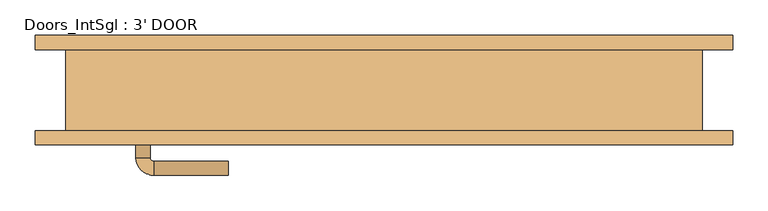
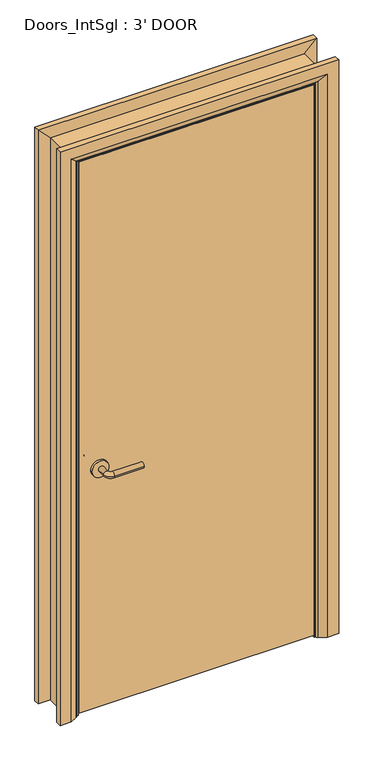
"""IFC4 building model written with IfcOpenShell, lengths in millimetres: door geometry, Doors_IntSgl : 3' DOOR."""

from ifc_helpers import new_model, si_unit, point, frame, frame_2d, origin, place, context, project, spatial, polyline, circle_curve, ellipse_curve, trimmed, segment, composite_curve, outline, extrude, faceted_brep, source, transform, mapped, element, save
from ifc_brep_helpers import plane_surface, cylinder_surface, revolved_surface, advanced_brep


def doors_intsgl_3_door_d2de26da(model_context):
    return source(origin(), model_context, "Body", "SolidModel", [
        advanced_brep(
        [(-350.2, -11.15, 900.0), (-330.2, -11.15, 900.0), (-350.2, 18.85, 900.0), (-330.2, 18.85, 900.0), (-325.2, 23.85, 900.0), (-325.2, 43.85, 900.0), (-220.2, 43.85, 900.0), (-220.2, 23.85, 900.0)],
        [
            (0, 1, circle_curve(frame((-340.2, -11.15, 900.0), z_axis=(0.0, -1.0, 0.0), x_axis=(1.0, 0.0, 0.0)), 10.0)),
            (1, 0, circle_curve(frame((-340.2, -11.15, 900.0), z_axis=(0.0, -1.0, 0.0), x_axis=(1.0, 0.0, 0.0)), 10.0)),
            (0, 2),
            (2, 3, circle_curve(frame((-340.2, 18.85, 900.0), z_axis=(0.0, -1.0, 0.0), x_axis=(1.0, 0.0, 0.0)), 10.0)),
            (3, 1),
            (3, 2, circle_curve(frame((-340.2, 18.85, 900.0), z_axis=(0.0, -1.0, 0.0), x_axis=(1.0, 0.0, 0.0)), 10.0)),
            (4, 3, circle_curve(frame((-325.2, 18.85, 900.0), z_axis=(0.0, 0.0, 1.0), x_axis=(-1.0, 0.0, 0.0)), 5.0)),
            (2, 5, circle_curve(frame((-325.2, 18.85, 900.0), z_axis=(0.0, 0.0, -1.0), x_axis=(-1.0, 0.0, 0.0)), 25.0)),
            (5, 4, circle_curve(frame((-325.2, 33.85, 900.0), z_axis=(-1.0, 0.0, 0.0), x_axis=(0.0, -1.0, 0.0)), 10.0)),
            (4, 5, circle_curve(frame((-325.2, 33.85, 900.0), z_axis=(-1.0, 0.0, 0.0), x_axis=(0.0, -1.0, 0.0)), 10.0)),
            (6, 7, circle_curve(frame((-220.2, 33.85, 900.0), z_axis=(1.0, 0.0, 0.0), x_axis=(0.0, -1.0, 0.0)), 10.0)),
            (7, 6, circle_curve(frame((-220.2, 33.85, 900.0), z_axis=(1.0, 0.0, 0.0), x_axis=(0.0, -1.0, 0.0)), 10.0)),
            (5, 6),
            (7, 4),
        ],
        [
            plane_surface(frame((-340.2, -11.15, 900.0), z_axis=(0.0, -1.0, 0.0), x_axis=(0.0, 0.0, 1.0))),
            cylinder_surface(frame((-340.2, -11.15, 900.0), z_axis=(0.0, -1.0, 0.0), x_axis=(1.0, 0.0, 0.0)), 10.0),
            revolved_surface(trimmed(ellipse_curve(frame((-340.2, 18.85, 900.0), z_axis=(0.0, -1.0, 0.0), x_axis=(1.0, 0.0, 0.0)), 10.0, 10.0), [point((-350.2, 18.85, 900.0))], [point((-330.2, 18.85, 900.0))], True, "CARTESIAN"), (-325.2, 18.85, 900.0), (0.0, 0.0, -1.0)),
            revolved_surface(trimmed(ellipse_curve(frame((-340.2, 18.85, 900.0), z_axis=(0.0, -1.0, 0.0), x_axis=(1.0, 0.0, 0.0)), 10.0, 10.0), [point((-330.2, 18.85, 900.0))], [point((-350.2, 18.85, 900.0))], True, "CARTESIAN"), (-325.2, 18.85, 900.0), (0.0, 0.0, -1.0)),
            plane_surface(frame((-220.2, 33.85, 900.0), z_axis=(1.0, 0.0, 0.0), x_axis=(0.0, 0.0, 1.0))),
            cylinder_surface(frame((-325.2, 33.85, 900.0), z_axis=(-1.0, 0.0, 0.0), x_axis=(0.0, -1.0, 0.0)), 10.0),
        ],
        [
            (0, [[1, 2]]),
            (1, [[-1, 3, 4, 5]]),
            (1, [[-2, -5, 6, -3]]),
            (2, [[7, -4, 8, 9]]),
            (3, [[-8, -6, -7, 10]]),
            (4, [[11, 12]]),
            (5, [[-9, 13, -12, 14]]),
            (5, [[-10, -14, -11, -13]]),
        ],
    ),
        extrude(outline(composite_curve([segment(trimmed(circle_curve(frame_2d((900.0, -342.7)), 30.0), [point((900.0, -372.7))], [point((900.0, -312.7))], False, "CARTESIAN"), True, "CONTINUOUS"), segment(trimmed(circle_curve(frame_2d((900.0, -342.7)), 30.0), [point((900.0, -312.7))], [point((900.0, -372.7))], False, "CARTESIAN"), True, "CONTINUOUS")], self_intersect=False)), frame((0.0, -19.15, 0.0), z_axis=(0.0, 1.0, 0.0), x_axis=(0.0, 0.0, 1.0)), (0.0, 0.0, 1.0), 8.0),
        advanced_brep(
        [(-350.2, -65.15, 900.0), (-330.2, -65.15, 900.0), (-330.2, -95.15, 900.0), (-350.2, -95.15, 900.0), (-325.2, -100.15, 900.0), (-325.2, -120.15, 900.0), (-220.2, -120.15, 900.0), (-220.2, -100.15, 900.0)],
        [
            (0, 1, circle_curve(frame((-340.2, -65.15, 900.0), z_axis=(0.0, 1.0, 0.0), x_axis=(1.0, 0.0, 0.0)), 10.0)),
            (1, 0, circle_curve(frame((-340.2, -65.15, 900.0), z_axis=(0.0, 1.0, 0.0), x_axis=(1.0, 0.0, 0.0)), 10.0)),
            (1, 2),
            (2, 3, circle_curve(frame((-340.2, -95.15, 900.0), z_axis=(0.0, 1.0, 0.0), x_axis=(1.0, 0.0, 0.0)), 10.0)),
            (3, 0),
            (3, 2, circle_curve(frame((-340.2, -95.15, 900.0), z_axis=(0.0, 1.0, 0.0), x_axis=(1.0, 0.0, 0.0)), 10.0)),
            (4, 5, circle_curve(frame((-325.2, -110.15, 900.0), z_axis=(-1.0, 0.0, 0.0), x_axis=(0.0, 1.0, 0.0)), 10.0)),
            (5, 3, circle_curve(frame((-325.2, -95.15, 900.0), z_axis=(0.0, 0.0, -1.0), x_axis=(-1.0, 0.0, 0.0)), 25.0)),
            (2, 4, circle_curve(frame((-325.2, -95.15, 900.0), z_axis=(0.0, 0.0, 1.0), x_axis=(-1.0, 0.0, 0.0)), 5.0)),
            (5, 4, circle_curve(frame((-325.2, -110.15, 900.0), z_axis=(-1.0, 0.0, 0.0), x_axis=(0.0, 1.0, 0.0)), 10.0)),
            (6, 7, circle_curve(frame((-220.2, -110.15, 900.0), z_axis=(1.0, 0.0, 0.0), x_axis=(0.0, 1.0, 0.0)), 10.0)),
            (7, 6, circle_curve(frame((-220.2, -110.15, 900.0), z_axis=(1.0, 0.0, 0.0), x_axis=(0.0, 1.0, 0.0)), 10.0)),
            (4, 7),
            (6, 5),
        ],
        [
            plane_surface(frame((-340.2, -65.15, 900.0), z_axis=(0.0, 1.0, 0.0), x_axis=(0.0, 0.0, 1.0))),
            cylinder_surface(frame((-340.2, -65.15, 900.0), z_axis=(0.0, 1.0, 0.0), x_axis=(1.0, 0.0, 0.0)), 10.0),
            revolved_surface(trimmed(ellipse_curve(frame((-340.2, -95.15, 900.0), z_axis=(0.0, -1.0, 0.0), x_axis=(1.0, 0.0, 0.0)), 10.0, 10.0), [point((-350.2, -95.15, 900.0))], [point((-330.2, -95.15, 900.0))], True, "CARTESIAN"), (-325.2, -95.15, 900.0), (0.0, 0.0, -1.0)),
            revolved_surface(trimmed(ellipse_curve(frame((-340.2, -95.15, 900.0), z_axis=(0.0, -1.0, 0.0), x_axis=(1.0, 0.0, 0.0)), 10.0, 10.0), [point((-330.2, -95.15, 900.0))], [point((-350.2, -95.15, 900.0))], True, "CARTESIAN"), (-325.2, -95.15, 900.0), (0.0, 0.0, -1.0)),
            plane_surface(frame((-220.2, -110.15, 900.0), z_axis=(1.0, 0.0, 0.0), x_axis=(0.0, 0.0, 1.0))),
            cylinder_surface(frame((-325.2, -110.15, 900.0), z_axis=(-1.0, 0.0, 0.0), x_axis=(0.0, 1.0, 0.0)), 10.0),
        ],
        [
            (0, [[1, 2]]),
            (1, [[3, 4, 5, -2]]),
            (1, [[-5, 6, -3, -1]]),
            (2, [[7, 8, -4, 9]]),
            (3, [[10, -9, -6, -8]]),
            (4, [[11, 12]]),
            (5, [[13, -11, 14, -7]]),
            (5, [[-14, -12, -13, -10]]),
        ],
    ),
        extrude(outline(composite_curve([segment(trimmed(circle_curve(frame_2d((900.0, -342.7)), 30.0), [point((900.0, -372.7))], [point((900.0, -312.7))], False, "CARTESIAN"), True, "CONTINUOUS"), segment(trimmed(circle_curve(frame_2d((900.0, -342.7)), 30.0), [point((900.0, -312.7))], [point((900.0, -372.7))], False, "CARTESIAN"), True, "CONTINUOUS")], self_intersect=False)), frame((0.0, -65.15, 0.0), z_axis=(0.0, 1.0, 0.0), x_axis=(0.0, 0.0, 1.0)), (0.0, 0.0, 1.0), 8.0),
        extrude(outline(polyline([(415.2, -19.15), (415.2, -57.15), (-415.2, -57.15), (-415.2, -19.15), (415.2, -19.15)])), frame((0.0, 0.0, 8.0), z_axis=(0.0, 0.0, 1.0), x_axis=(1.0, 0.0, 0.0)), (0.0, 0.0, 1.0), 2060.0),
        advanced_brep(
        [(492.2, -77.15, 0.0), (452.2, -77.15, 0.0), (426.2, -63.15, 0.0), (422.2, -57.15, 0.0), (492.2, -57.15, 0.0), (492.2, -57.15, 2145.0), (492.2, -77.15, 2145.0), (422.2, -57.15, 2075.0), (-422.2, -57.15, 2075.0), (-422.2, -57.15, 0.0), (-492.2, -57.15, 0.0), (-492.2, -57.15, 2145.0), (426.2, -63.15, 2079.0), (452.2, -77.15, 2105.0), (-492.2, -77.15, 2145.0), (-492.2, -77.15, 0.0), (-452.2, -77.15, 0.0), (-452.2, -77.15, 2105.0), (-426.2, -63.15, 0.0), (-426.2, -63.15, 2079.0)],
        [
            (0, 1),
            (1, 2),
            (2, 3, circle_curve(frame((430.2, -56.15, 0.0), z_axis=(0.0, 0.0, -1.0), x_axis=(1.0, 0.0, 0.0)), 8.0622577)),
            (3, 4),
            (4, 0),
            (4, 5),
            (5, 6),
            (6, 0),
            (3, 7),
            (7, 8),
            (8, 9),
            (9, 10),
            (10, 11),
            (11, 5),
            (2, 12),
            (12, 7, ellipse_curve(frame((430.2, -56.15, 2083.0), z_axis=(0.7071067811865475, 0.0, -0.7071067811865475), x_axis=(-0.7071067811865474, 0.0, -0.7071067811865476)), 11.4017543, 8.0622577)),
            (1, 13),
            (13, 12),
            (6, 14),
            (14, 15),
            (15, 16),
            (16, 17),
            (17, 13),
            (10, 15),
            (14, 11),
            (9, 18, circle_curve(frame((-430.2, -56.15, 0.0), z_axis=(0.0, 0.0, -1.0), x_axis=(-1.0, 0.0, 0.0)), 8.0622577)),
            (18, 16),
            (19, 18),
            (8, 19, ellipse_curve(frame((-430.2, -56.15, 2083.0), z_axis=(-0.7071067811865475, 0.0, -0.7071067811865475), x_axis=(-0.7071067811865474, 0.0, 0.7071067811865476)), 11.4017543, 8.0622577)),
            (19, 17),
            (12, 19),
        ],
        [
            plane_surface(frame((422.2, -57.15, 0.0), z_axis=(0.0, 0.0, -1.0), x_axis=(0.0, 1.0, 0.0))),
            plane_surface(frame((492.2, -77.15, 0.0), z_axis=(1.0, 0.0, 0.0), x_axis=(0.0, 0.0, 1.0))),
            plane_surface(frame((492.2, -57.15, 0.0), z_axis=(0.0, 1.0, 0.0), x_axis=(0.0, 0.0, 1.0))),
            cylinder_surface(frame((430.2, -56.15, 0.0), z_axis=(0.0, 0.0, -1.0), x_axis=(1.0, 0.0, 0.0)), 8.0622577),
            plane_surface(frame((426.2, -63.15, 0.0), z_axis=(-0.4740998230350126, -0.880471099922178, 0.0), x_axis=(0.0, 0.0, 1.0))),
            plane_surface(frame((452.2, -77.15, 0.0), z_axis=(0.0, -1.0, 0.0), x_axis=(0.0, 0.0, 1.0))),
            plane_surface(frame((-492.2, -77.15, 2145.0), z_axis=(-1.0, 0.0, 0.0), x_axis=(0.0, 0.0, -1.0))),
            plane_surface(frame((-422.2, -57.15, 0.0), z_axis=(0.0, 0.0, -1.0), x_axis=(0.0, 1.0, 0.0))),
            cylinder_surface(frame((-430.2, -56.15, 2075.0), z_axis=(0.0, 0.0, 1.0), x_axis=(-1.0, 0.0, 0.0)), 8.0622577),
            plane_surface(frame((-426.2, -63.15, 2079.0), z_axis=(0.47409982303501824, -0.8804710999221749, 0.0), x_axis=(0.0, 0.0, -1.0))),
            plane_surface(frame((492.2, -77.15, 2145.0), z_axis=(0.0, 0.0, 1.0), x_axis=(-1.0, 0.0, 0.0))),
            cylinder_surface(frame((422.2, -56.15, 2083.0), z_axis=(1.0, 0.0, 0.0), x_axis=(0.0, 0.0, 1.0)), 8.0622577),
            plane_surface(frame((426.2, -63.15, 2079.0), z_axis=(0.0, -0.8804710999221764, -0.4740998230350154), x_axis=(-1.0, 0.0, 0.0))),
        ],
        [
            (0, [[1, 2, 3, 4, 5]]),
            (1, [[6, 7, 8, -5]]),
            (2, [[9, 10, 11, 12, 13, 14, -6, -4]]),
            (3, [[15, 16, -9, -3]]),
            (4, [[17, 18, -15, -2]]),
            (5, [[-8, 19, 20, 21, 22, 23, -17, -1]]),
            (6, [[-13, 24, -20, 25]]),
            (7, [[-24, -12, 26, 27, -21]]),
            (8, [[28, -26, -11, 29]]),
            (9, [[-22, -27, -28, 30]]),
            (10, [[-14, -25, -19, -7]]),
            (11, [[31, -29, -10, -16]]),
            (12, [[-23, -30, -31, -18]]),
        ],
    ),
        extrude(outline(polyline([(0.0, -398.2), (2051.0, -398.2), (2051.0, 398.2), (0.0, 398.2), (0.0, 417.2), (2070.0, 417.2), (2070.0, -417.2), (0.0, -417.2), (0.0, -398.2)])), frame((0.0, -17.15, 0.0), z_axis=(0.0, 1.0, 0.0), x_axis=(0.0, 0.0, 1.0)), (0.0, 0.0, 1.0), 32.0),
        advanced_brep(
        [(-492.2, 77.15, 0.0), (-452.2, 77.15, 0.0), (-426.2, 63.15, 0.0), (-422.2, 57.15, 0.0), (-492.2, 57.15, 0.0), (-492.2, 57.15, 2145.0), (-492.2, 77.15, 2145.0), (-422.2, 57.15, 2075.0), (-426.2, 63.15, 2079.0), (-452.2, 77.15, 2105.0), (492.2, 77.15, 0.0), (492.2, 57.15, 0.0), (422.2, 57.15, 0.0), (426.2, 63.15, 0.0), (452.2, 77.15, 0.0), (492.2, 77.15, 2145.0), (452.2, 77.15, 2105.0), (426.2, 63.15, 2079.0), (422.2, 57.15, 2075.0), (492.2, 57.15, 2145.0)],
        [
            (0, 1),
            (1, 2),
            (2, 3, circle_curve(frame((-430.2, 56.15, 0.0), z_axis=(0.0, 0.0, -1.0), x_axis=(-1.0, 0.0, 0.0)), 8.0622577)),
            (3, 4),
            (4, 0),
            (4, 5),
            (5, 6),
            (6, 0),
            (3, 7),
            (7, 5),
            (2, 8),
            (8, 7, ellipse_curve(frame((-430.2, 56.15, 2083.0), z_axis=(-0.7071067811865475, 0.0, -0.7071067811865475), x_axis=(0.7071067811865474, 0.0, -0.7071067811865476)), 11.4017543, 8.0622577)),
            (1, 9),
            (9, 8),
            (6, 9),
            (10, 11),
            (11, 12),
            (12, 13, circle_curve(frame((430.2, 56.15, 0.0), z_axis=(0.0, 0.0, -1.0), x_axis=(1.0, 0.0, 0.0)), 8.0622577)),
            (13, 14),
            (14, 10),
            (15, 10),
            (14, 16),
            (16, 15),
            (13, 17),
            (17, 16),
            (12, 18),
            (18, 17, ellipse_curve(frame((430.2, 56.15, 2083.0), z_axis=(0.7071067811865475, 0.0, -0.7071067811865475), x_axis=(0.7071067811865474, 0.0, 0.7071067811865476)), 11.4017543, 8.0622577)),
            (11, 19),
            (19, 18),
            (15, 19),
            (5, 19),
            (15, 6),
            (7, 18),
            (8, 17),
            (9, 16),
        ],
        [
            plane_surface(frame((-422.2, 129.9510989, 0.0), z_axis=(0.0, 0.0, -1.0), x_axis=(1.0, 0.0, 0.0))),
            plane_surface(frame((-492.2, 77.15, 0.0), z_axis=(-1.0, 0.0, 0.0), x_axis=(0.0, 0.0, 1.0))),
            plane_surface(frame((-492.2, 57.15, 0.0), z_axis=(0.0, -1.0, 0.0), x_axis=(0.0, 0.0, 1.0))),
            cylinder_surface(frame((-430.2, 56.15, 0.0), z_axis=(0.0, 0.0, -1.0), x_axis=(-1.0, 0.0, 0.0)), 8.0622577),
            plane_surface(frame((-426.2, 63.15, 0.0), z_axis=(0.4740998230350183, 0.8804710999221749, 0.0), x_axis=(0.0, 0.0, 1.0))),
            plane_surface(frame((-452.2, 77.15, 0.0), z_axis=(0.0, 1.0, 0.0), x_axis=(0.0, 0.0, 1.0))),
            plane_surface(frame((422.2, 129.9510989, 0.0), z_axis=(0.0, 0.0, -1.0), x_axis=(-1.0, 0.0, 0.0))),
            plane_surface(frame((452.2, 77.15, 2105.0), z_axis=(0.0, 1.0, 0.0), x_axis=(0.0, 0.0, -1.0))),
            plane_surface(frame((426.2, 63.15, 2079.0), z_axis=(-0.4740998230350183, 0.8804710999221749, 0.0), x_axis=(0.0, 0.0, -1.0))),
            cylinder_surface(frame((430.2, 56.15, 2075.0), z_axis=(0.0, 0.0, 1.0), x_axis=(1.0, 0.0, 0.0)), 8.0622577),
            plane_surface(frame((492.2, 57.15, 2145.0), z_axis=(0.0, -1.0, 0.0), x_axis=(0.0, 0.0, -1.0))),
            plane_surface(frame((492.2, 77.15, 2145.0), z_axis=(1.0, 0.0, 0.0), x_axis=(0.0, 0.0, -1.0))),
            plane_surface(frame((-492.2, 77.15, 2145.0), z_axis=(0.0, 0.0, 1.0), x_axis=(1.0, 0.0, 0.0))),
            plane_surface(frame((-492.2, 57.15, 2145.0), z_axis=(0.0, -1.0, 0.0), x_axis=(1.0, 0.0, 0.0))),
            cylinder_surface(frame((-422.2, 56.15, 2083.0), z_axis=(-1.0, 0.0, 0.0), x_axis=(0.0, 0.0, 1.0)), 8.0622577),
            plane_surface(frame((-426.2, 63.15, 2079.0), z_axis=(0.0, 0.8804710999221749, -0.4740998230350183), x_axis=(1.0, 0.0, 0.0))),
            plane_surface(frame((-452.2, 77.15, 2105.0), z_axis=(0.0, 1.0, 0.0), x_axis=(1.0, 0.0, 0.0))),
        ],
        [
            (0, [[1, 2, 3, 4, 5]]),
            (1, [[6, 7, 8, -5]]),
            (2, [[9, 10, -6, -4]]),
            (3, [[11, 12, -9, -3]]),
            (4, [[13, 14, -11, -2]]),
            (5, [[-8, 15, -13, -1]]),
            (6, [[16, 17, 18, 19, 20]]),
            (7, [[21, -20, 22, 23]]),
            (8, [[-22, -19, 24, 25]]),
            (9, [[-24, -18, 26, 27]]),
            (10, [[-26, -17, 28, 29]]),
            (11, [[-28, -16, -21, 30]]),
            (12, [[31, -30, 32, -7]]),
            (13, [[33, -29, -31, -10]]),
            (14, [[34, -27, -33, -12]]),
            (15, [[35, -25, -34, -14]]),
            (16, [[-32, -23, -35, -15]]),
        ],
    ),
        faceted_brep([(-417.2, -57.15, 0.0), (-449.2, -57.15, 0.0), (-449.2, 57.15, 0.0), (-417.2, 57.15, 0.0), (-417.2, 57.15, 2070.0), (-417.2, -57.15, 2070.0), (-449.2, 57.15, 2102.0), (-449.2, -57.15, 2102.0), (417.2, -57.15, 0.0), (417.2, 57.15, 0.0), (449.2, 57.15, 0.0), (449.2, -57.15, 0.0), (417.2, -57.15, 2070.0), (449.2, -57.15, 2102.0), (449.2, 57.15, 2102.0), (417.2, 57.15, 2070.0)], [[[0, 1, 2, 3]], [[3, 4, 5, 0]], [[2, 6, 4, 3]], [[1, 7, 6, 2]], [[0, 5, 7, 1]], [[8, 9, 10, 11]], [[12, 8, 11, 13]], [[13, 11, 10, 14]], [[14, 10, 9, 15]], [[15, 9, 8, 12]], [[4, 15, 12, 5]], [[6, 14, 15, 4]], [[7, 13, 14, 6]], [[5, 12, 13, 7]]]),
    ])


if __name__ == "__main__":
    model = new_model("IFC4")
    model_context = context("Model", 3, world=origin())
    ifc_project = project(units=[si_unit("LENGTHUNIT", "METRE", prefix="MILLI")], contexts=[model_context])
    site = spatial("IfcSite", under=ifc_project)
    building = spatial("IfcBuilding", under=site)
    placement = place(None, origin())
    doors_intsgl_3_door_shape = doors_intsgl_3_door_d2de26da(model_context)
    element("IfcDoor", 1, ObjectType="Doors_IntSgl : 3' DOOR", at=placement, inside=building, context=model_context, shape_type="MappedRepresentation", body=[
        mapped(doors_intsgl_3_door_shape, transform((0.0, 0.0, 0.0), x_axis=(1.0, 0.0, 0.0), y_axis=(0.0, 1.0, 0.0), z_axis=(0.0, 0.0, 1.0))),
    ])
    save(model, "model.ifc")

# Revit data of these elements
# Type "Doors_IntSgl : 3' DOOR"
#   Type Mark = "46"
#   Type Comments = "Internal Single"
#   Operation = "SingleSwingRight"
#   Manufacturer = "Revit"
#   Keynote = "L20"
#   Description = "Internal Single Door"
#   Analytic Construction = "Metal"
#   UnderCut = 0.026247 ft
#   Tolerance = 0.006562 ft
#   Thickness = 0.124672 ft
#   Thermal Resistance (R) = 0.270117 (m²·K)/W
#   Structural Tolerance = 0.026247 ft
#   StopDepth = 0.104987 ft
#   Stop Thickness = 0.062336 ft
#   Rough Width = 3.0 ft
#   Rough Height = 6.922572 ft
#   Height to Top Lock Rail = 3.28084 ft
#   Heat Transfer Coefficient (U) = 3.7021 W/(m²·K)
#   Handle Z Distance = 2.952756 ft
#   Handle X Distance = 0.246063 ft
#   Frame Thickness = 0.104987 ft
#   Door Panel Width = 2.724409 ft
#   Door Panel Thickness = 0.124672 ft
#   Door Panel Offset = 0.0 ft
#   Height = 6.922572 ft
#   Width = 3.0 ft
#   Door Panel Height = 6.75853 ft
#   Architrave Setback = 0.016404 ft
#   Vis - Ironmongery = yes
#   Material Ironmongery = Door - Handle
#   Material Frame = Door - Frame/Mullion (1)
#   Material Door = Door - Panel
#   Material Architrave = Door - Architrave
#   Visual Light Transmittance = 0
#   Solar Heat Gain Coefficient = 0
#   Function = (empty or 0)
#   Wall Closure = (empty or 0)
# Element 1 (IfcDoor, "Doors_IntSgl : 3' DOOR")
#   Materials on its faces: "Door - Architrave", "Door - Handle", "Door - Frame/Mullion (1)", "Door - Panel"
# Materials
#   "Door - Handle": colour RGB 0 0 0, transparency 0, Keynote = "P21", Cost = 0
#   "Door - Frame/Mullion (1)": class "Wood", colour RGB 212 179 113, transparency 0, Keynote = "L20", Cost = 0
#   "Door - Panel": class "Wood", colour RGB 210 159 95, transparency 0, Keynote = "L20", Cost = 0
#   "Door - Architrave": class "Wood", colour RGB 154 90 5, transparency 0, Keynote = "P20", Cost = 0
